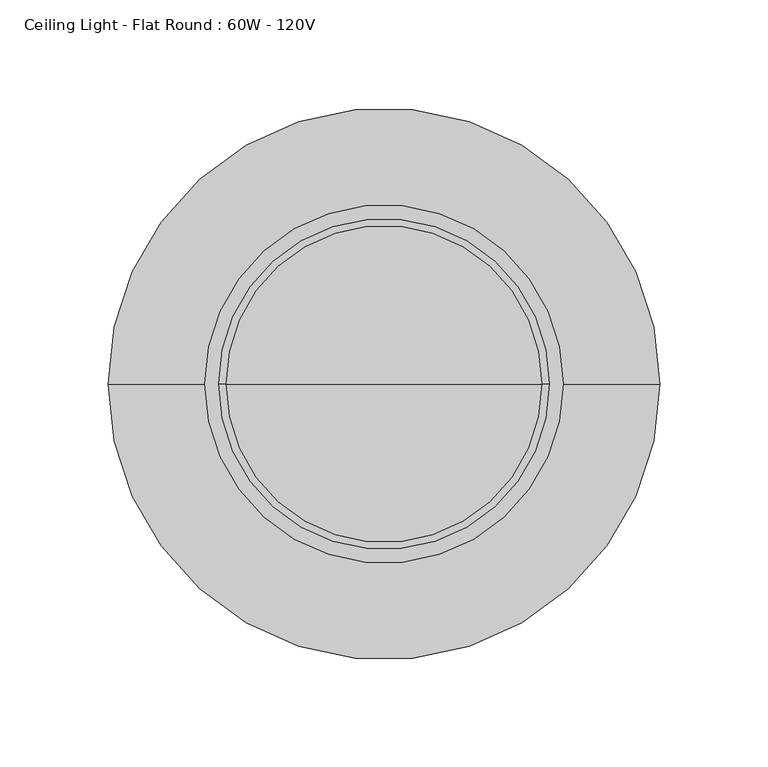
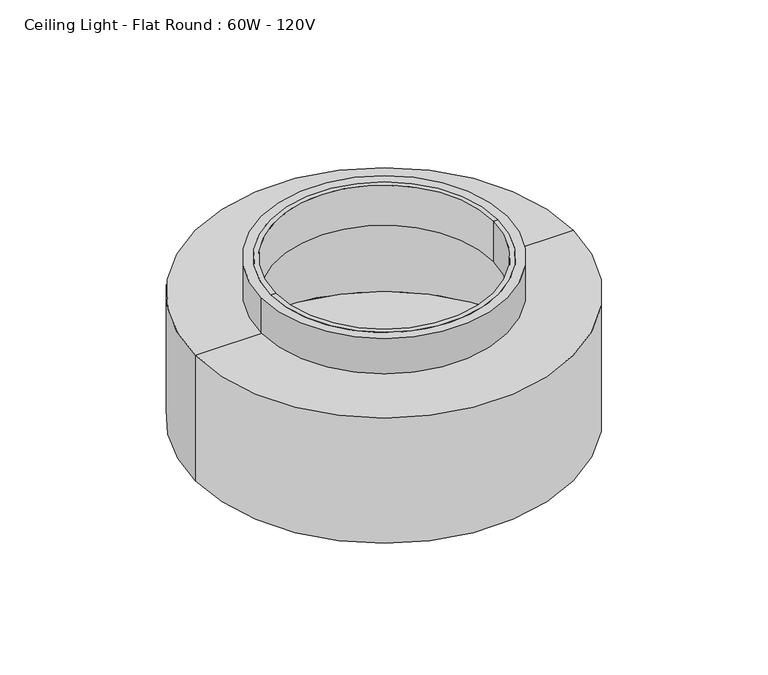
"""IFC4 building model written with IfcOpenShell, lengths in millimetres: light fixture geometry, Ceiling Light - Flat Round : 60W - 120V."""

from ifc_helpers import new_model, si_unit, point, frame, origin, origin_2d, place, context, project, spatial, polyline, circle_curve, trimmed, segment, composite_curve, outline, extrude, source, transform, mapped, element, save
from ifc_brep_helpers import plane_surface, cylinder_surface, revolved_surface, advanced_brep


def ceiling_light_flat_round_60w_120v_7c4c2a52(model_context):
    return source(origin(), model_context, "Body", "SolidModel", [
        advanced_brep(
        [(127.0, 0.0, 2413.0), (-127.0, 0.0, 2413.0), (-76.2, 0.0, 2413.0), (76.2, 0.0, 2413.0), (127.0, 0.0, 2324.1), (-127.0, 0.0, 2324.1), (0.0, 0.0, 2324.1), (123.825, 0.0, 2327.275), (-123.825, 0.0, 2327.275), (0.0, 0.0, 2327.275), (123.825, 0.0, 2409.825), (-123.825, 0.0, 2409.825), (73.025, 0.0, 2409.825), (-73.025, 0.0, 2409.825), (73.025, 0.0, 2438.4), (-73.025, 0.0, 2438.4), (76.2, 0.0, 2438.4), (-76.2, 0.0, 2438.4)],
        [
            (0, 1, circle_curve(frame((0.0, 0.0, 2413.0), z_axis=(0.0, 0.0, 1.0), x_axis=(-1.0, 0.0, 0.0)), 127.0)),
            (1, 2),
            (2, 3, circle_curve(frame((0.0, 0.0, 2413.0), z_axis=(0.0, 0.0, -1.0), x_axis=(-1.0, 0.0, 0.0)), 76.2)),
            (3, 0),
            (1, 0, circle_curve(frame((0.0, 0.0, 2413.0), z_axis=(0.0, 0.0, 1.0), x_axis=(-1.0, 0.0, 0.0)), 127.0)),
            (3, 2, circle_curve(frame((0.0, 0.0, 2413.0), z_axis=(0.0, 0.0, -1.0), x_axis=(-1.0, 0.0, 0.0)), 76.2)),
            (4, 5, circle_curve(frame((0.0, 0.0, 2324.1), z_axis=(0.0, 0.0, 1.0), x_axis=(-1.0, 0.0, 0.0)), 127.0)),
            (5, 1),
            (0, 4),
            (5, 4, circle_curve(frame((0.0, 0.0, 2324.1), z_axis=(0.0, 0.0, 1.0), x_axis=(-1.0, 0.0, 0.0)), 127.0)),
            (6, 5),
            (4, 6),
            (7, 8, circle_curve(frame((0.0, 0.0, 2327.275), z_axis=(0.0, 0.0, 1.0), x_axis=(-1.0, 0.0, 0.0)), 123.825)),
            (8, 9),
            (9, 7),
            (8, 7, circle_curve(frame((0.0, 0.0, 2327.275), z_axis=(0.0, 0.0, 1.0), x_axis=(-1.0, 0.0, 0.0)), 123.825)),
            (10, 11, circle_curve(frame((0.0, 0.0, 2409.825), z_axis=(0.0, 0.0, 1.0), x_axis=(-1.0, 0.0, 0.0)), 123.825)),
            (11, 8),
            (7, 10),
            (11, 10, circle_curve(frame((0.0, 0.0, 2409.825), z_axis=(0.0, 0.0, 1.0), x_axis=(-1.0, 0.0, 0.0)), 123.825)),
            (12, 13, circle_curve(frame((0.0, 0.0, 2409.825), z_axis=(0.0, 0.0, 1.0), x_axis=(-1.0, 0.0, 0.0)), 73.025)),
            (13, 11),
            (10, 12),
            (13, 12, circle_curve(frame((0.0, 0.0, 2409.825), z_axis=(0.0, 0.0, 1.0), x_axis=(-1.0, 0.0, 0.0)), 73.025)),
            (14, 15, circle_curve(frame((0.0, 0.0, 2438.4), z_axis=(0.0, 0.0, 1.0), x_axis=(-1.0, 0.0, 0.0)), 73.025)),
            (15, 13),
            (12, 14),
            (15, 14, circle_curve(frame((0.0, 0.0, 2438.4), z_axis=(0.0, 0.0, 1.0), x_axis=(-1.0, 0.0, 0.0)), 73.025)),
            (16, 17, circle_curve(frame((0.0, 0.0, 2438.4), z_axis=(0.0, 0.0, 1.0), x_axis=(-1.0, 0.0, 0.0)), 76.2)),
            (17, 15),
            (14, 16),
            (17, 16, circle_curve(frame((0.0, 0.0, 2438.4), z_axis=(0.0, 0.0, 1.0), x_axis=(-1.0, 0.0, 0.0)), 76.2)),
            (2, 17),
            (16, 3),
        ],
        [
            plane_surface(frame((0.0, 0.0, 2413.0), z_axis=(0.0, 0.0, 1.0), x_axis=(-1.0, 0.0, 0.0))),
            cylinder_surface(frame((0.0, 0.0, 2463.8), z_axis=(0.0, 0.0, -1.0), x_axis=(-1.0, 0.0, 0.0)), 127.0),
            plane_surface(frame((0.0, 0.0, 2324.1), z_axis=(0.0, 0.0, -1.0), x_axis=(-1.0, 0.0, 0.0))),
            plane_surface(frame((0.0, 0.0, 2327.275), z_axis=(0.0, 0.0, 1.0), x_axis=(-1.0, 0.0, 0.0))),
            revolved_surface(polyline([(-123.825, 0.0, 2327.275), (-123.825, 0.0, 2409.825)]), (0.0, 0.0, 2463.8), (0.0, 0.0, -1.0)),
            plane_surface(frame((0.0, 0.0, 2409.825), z_axis=(0.0, 0.0, -1.0), x_axis=(-1.0, 0.0, 0.0))),
            revolved_surface(polyline([(-73.025, 0.0, 2409.825), (-73.025, 0.0, 2438.4)]), (0.0, 0.0, 2463.8), (0.0, 0.0, -1.0)),
            plane_surface(frame((0.0, 0.0, 2438.4), z_axis=(0.0, 0.0, 1.0), x_axis=(-1.0, 0.0, 0.0))),
            cylinder_surface(frame((0.0, 0.0, 2463.8), z_axis=(0.0, 0.0, -1.0), x_axis=(-1.0, 0.0, 0.0)), 76.2),
        ],
        [
            (0, [[1, 2, 3, 4]]),
            (0, [[5, -4, 6, -2]]),
            (1, [[7, 8, -1, 9]]),
            (1, [[10, -9, -5, -8]]),
            (2, [[11, -7, 12]]),
            (2, [[-12, -10, -11]]),
            (3, [[13, 14, 15]]),
            (3, [[16, -15, -14]]),
            (4, [[17, 18, -13, 19]]),
            (4, [[20, -19, -16, -18]]),
            (5, [[21, 22, -17, 23]]),
            (5, [[24, -23, -20, -22]]),
            (6, [[25, 26, -21, 27]]),
            (6, [[28, -27, -24, -26]]),
            (7, [[29, 30, -25, 31]]),
            (7, [[32, -31, -28, -30]]),
            (8, [[-3, 33, -29, 34]]),
            (8, [[-6, -34, -32, -33]]),
        ],
    ),
        extrude(outline(composite_curve([segment(trimmed(circle_curve(origin_2d(), 82.55), [point((-82.55, 0.0))], [point((82.55, 0.0))], False, "CARTESIAN"), True, "CONTINUOUS"), segment(trimmed(circle_curve(origin_2d(), 82.55), [point((82.55, 0.0))], [point((-82.55, 0.0))], False, "CARTESIAN"), True, "CONTINUOUS")], self_intersect=False), holes=[composite_curve([segment(trimmed(circle_curve(origin_2d(), 76.2), [point((-76.2, 0.0))], [point((76.2, 0.0))], True, "CARTESIAN"), True, "CONTINUOUS"), segment(trimmed(circle_curve(origin_2d(), 76.2), [point((76.2, 0.0))], [point((-76.2, 0.0))], True, "CARTESIAN"), True, "CONTINUOUS")], self_intersect=False)]), frame((0.0, 0.0, 2413.0), z_axis=(0.0, 0.0, 1.0), x_axis=(1.0, 0.0, 0.0)), (0.0, 0.0, 1.0), 25.4),
    ])


if __name__ == "__main__":
    model = new_model("IFC4")
    model_context = context("Model", 3, world=origin())
    ifc_project = project(units=[si_unit("LENGTHUNIT", "METRE", prefix="MILLI")], contexts=[model_context])
    site = spatial("IfcSite", under=ifc_project)
    building = spatial("IfcBuilding", under=site)
    placement = place(None, origin())
    ceiling_light_flat_round_60w_120v_shape = ceiling_light_flat_round_60w_120v_7c4c2a52(model_context)
    element("IfcLightFixture", 1, ObjectType="Ceiling Light - Flat Round : 60W - 120V", at=placement, inside=building, context=model_context, shape_type="MappedRepresentation", body=[
        mapped(ceiling_light_flat_round_60w_120v_shape, transform((0.0, 0.0, 0.0), x_axis=(1.0, 0.0, 0.0), y_axis=(0.0, 1.0, 0.0), z_axis=(0.0, 0.0, 1.0))),
    ])
    save(model, "model.ifc")

# Revit data of these elements
# Type "Ceiling Light - Flat Round : 60W - 120V"
#   Lamp = "A-19"
#   Assembly Code = "D5020220"
#   Wattage = 60 W
#   built-in parameter 1150110 = 1 (stored number, unit not read)
#   built-in parameter 1114217 = 1 (stored number, unit not read)
#   built-in parameter 1150109 = 1 (stored number, unit not read)
#   built-in parameter 1150113 = 1 (stored number, unit not read)
#   built-in parameter 1150115 = 1 (stored number, unit not read)
#   built-in parameter 1150105 = 272.155 (stored number, unit not read)
#   Light Source Symbol Size = 2' - 0"
#   built-in parameter 1150112 = 1 (stored number, unit not read)
#   built-in parameter 1150114 = 1 (stored number, unit not read)
#   built-in parameter 1150107 = 2800 (stored number, unit not read)
#   built-in parameter 1150106 = 2.72155 (stored number, unit not read)
#   Emit from Circle Diameter = 0' - 10"
#   built-in parameter 1150104 = 1.32387 (stored number, unit not read)
#   Ballast Voltage = 120 V
#   built-in parameter 1114218 = 1 (stored number, unit not read)
#   built-in parameter 1150133 = 10 (stored number, unit not read)
#   Lumens = 855 lm
#   Apparent Load = 60 VA
#   built-in parameter 1150134 = 4
#   built-in parameter 1150137 = 1
#   Color Filter = 16777215
#   built-in parameter 1140040 [instance default] = 1
#   Ballast Number of Poles = 1
#   Light Box Material = Steel, Paint Finish, Dark Gray, Matte
#   Diffuser Material = Glass, White, High Luminance
#   Wattage Comments = ""
#   Emit Shape Visible in Rendering = no
#   Dimming Lamp Color Temperature Shift = (empty or 0)
#   Default Elevation = 0
# Element 1 (IfcLightFixture, "Ceiling Light - Flat Round : 60W - 120V")
#   Materials on its faces: "Glass, White, High Luminance", "Steel, Paint Finish, Dark Gray, Matte"
# Materials
#   "Steel, Paint Finish, Dark Gray, Matte": class "Metal", colour RGB 98 98 98, transparency 0, Description = "Steel, paint finish, dark gray, matte", Cost = 0
#   "Glass, White, High Luminance": class "Glass", colour RGB 249 250 249, transparency 0.8, Description = "physical material", Cost = 0
